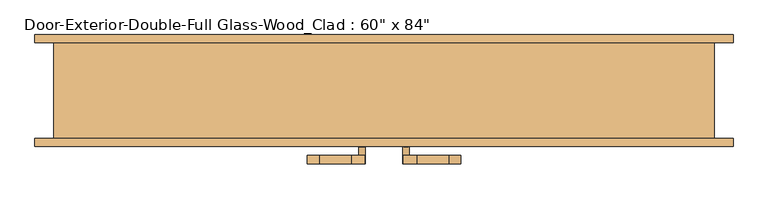
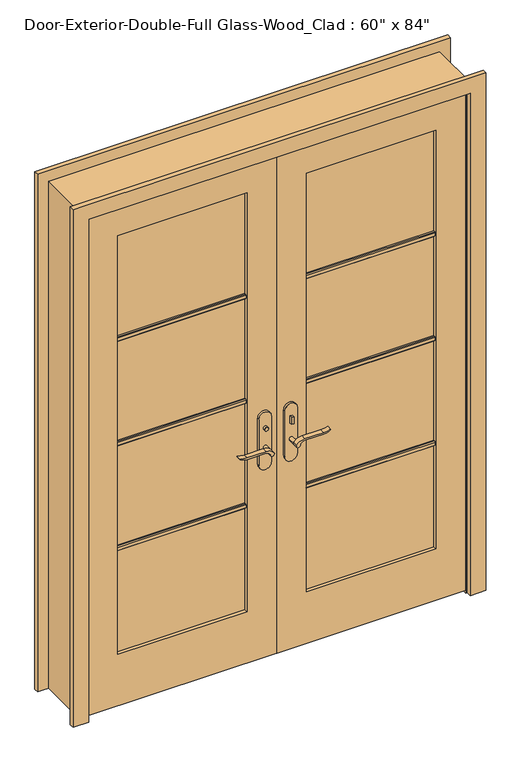
"""IFC4 building model written with IfcOpenShell, lengths in millimetres: door geometry."""

from ifc_helpers import new_model, si_unit, point, frame, frame_2d, origin, place, context, project, spatial, polyline, circle_curve, trimmed, segment, composite_curve, outline, extrude, faceted_brep, source, transform, mapped, element, save


def door_7bc300fe(model_context):
    return source(origin(), model_context, "Body", "SolidModel", [
        extrude(outline(polyline([(-19.05, 12.7), (6.35, 0.0), (-79.375, 0.0), (-53.975, 12.7), (-19.05, 12.7)])), frame((-762.0, 0.0, 0.0), z_axis=(1.0, 0.0, 0.0), x_axis=(0.0, 1.0, 0.0)), (0.0, 0.0, 1.0), 1524.0),
        extrude(outline(polyline([(-47.4019111, -56.2), (-47.4019111, -66.2), (-57.4019111, -66.2), (-57.4019111, -56.2), (-47.4019111, -56.2)])), frame((0.0, 0.0, 981.9), z_axis=(0.0, 0.0, 1.0), x_axis=(1.0, 0.0, 0.0)), (0.0, 0.0, 1.0), 30.0),
        extrude(outline(composite_curve([segment(trimmed(circle_curve(frame_2d((996.9, -52.4019111)), 8.0), [point((996.9, -60.4019111))], [point((996.9, -44.4019111))], False, "CARTESIAN"), True, "CONTINUOUS"), segment(trimmed(circle_curve(frame_2d((996.9, -52.4019111)), 8.0), [point((996.9, -44.4019111))], [point((996.9, -60.4019111))], False, "CARTESIAN"), True, "CONTINUOUS")], self_intersect=False)), frame((0.0, -131.125, 0.0), z_axis=(0.0, 1.0, 0.0), x_axis=(0.0, 0.0, 1.0)), (0.0, 0.0, 1.0), 10.0),
        extrude(outline(composite_curve([segment(trimmed(circle_curve(frame_2d((897.1555521, -76.0694241)), 37.2832219), [point((919.0523287, -45.8937749))], [point((934.4, -77.7693445))], False, "CARTESIAN"), True, "CONTINUOUS"), segment(polyline([(934.4, -77.7693445), (934.4, -154.045502)]), True, "CONTINUOUS"), segment(trimmed(circle_curve(frame_2d((1017.6850638, -153.9791202)), 83.2850902), [point((934.4, -154.045502))], [point((939.4, -182.4019111))], True, "CARTESIAN"), True, "CONTINUOUS"), segment(polyline([(939.4, -182.4019111), (936.6135558, -182.4019111)]), True, "CONTINUOUS"), segment(trimmed(circle_curve(frame_2d((986.6709207, -150.4622499)), 59.3791355), [point((936.6135558, -182.4019111))], [point((927.4, -154.045502))], False, "CARTESIAN"), True, "CONTINUOUS"), segment(polyline([(927.4, -154.045502), (927.4, -77.7881013)]), True, "CONTINUOUS"), segment(trimmed(circle_curve(frame_2d((909.2738613, -77.7881013)), 18.1261387), [point((927.4, -77.7881013))], [point((914.4, -60.4019111))], True, "CARTESIAN"), True, "CONTINUOUS"), segment(trimmed(circle_curve(frame_2d((914.4, -52.4019111)), 8.0), [point((914.4, -60.4019111))], [point((919.0523287, -45.8937749))], False, "CARTESIAN"), True, "CONTINUOUS")], self_intersect=False)), frame((0.0, -36.2, 0.0), z_axis=(0.0, 1.0, 0.0), x_axis=(0.0, 0.0, 1.0)), (0.0, 0.0, 1.0), 20.0),
        extrude(outline(composite_curve([segment(trimmed(circle_curve(frame_2d((914.4, -52.4019111)), 8.0), [point((914.3999903, -60.4019111))], [point((919.0523287, -45.8937749))], False, "CARTESIAN"), True, "CONTINUOUS"), segment(trimmed(circle_curve(frame_2d((897.1555521, -76.0694241)), 37.2832219), [point((919.0523287, -45.8937749))], [point((934.4, -77.7693445))], False, "CARTESIAN"), True, "CONTINUOUS"), segment(polyline([(934.4, -77.7693445), (934.4, -154.045502)]), True, "CONTINUOUS"), segment(trimmed(circle_curve(frame_2d((1017.6850638, -153.9791202)), 83.2850902), [point((934.4, -154.045502))], [point((939.4, -182.4019111))], True, "CARTESIAN"), True, "CONTINUOUS"), segment(polyline([(939.4, -182.4019111), (936.6135558, -182.4019111)]), True, "CONTINUOUS"), segment(trimmed(circle_curve(frame_2d((986.6709207, -150.4622499)), 59.3791355), [point((936.6135558, -182.4019111))], [point((927.4, -154.045502))], False, "CARTESIAN"), True, "CONTINUOUS"), segment(polyline([(927.4, -154.045502), (927.4, -77.788099)]), True, "CONTINUOUS"), segment(trimmed(circle_curve(frame_2d((909.2738682, -77.788099)), 18.1261318), [point((927.4, -77.788099))], [point((914.3999903, -60.4019111))], True, "CARTESIAN"), True, "CONTINUOUS")], self_intersect=False)), frame((0.0, -171.125, 0.0), z_axis=(0.0, 1.0, 0.0), x_axis=(0.0, 0.0, 1.0)), (0.0, 0.0, 1.0), 20.0),
        extrude(outline(composite_curve([segment(trimmed(circle_curve(frame_2d((914.4, -52.4019111)), 8.0), [point((914.4, -60.4019111))], [point((914.4, -44.4019111))], False, "CARTESIAN"), True, "CONTINUOUS"), segment(trimmed(circle_curve(frame_2d((914.4, -52.4019111)), 8.0), [point((914.4, -44.4019111))], [point((914.4, -60.4019111))], False, "CARTESIAN"), True, "CONTINUOUS")], self_intersect=False)), frame((0.0, -66.2, 0.0), z_axis=(0.0, 1.0, 0.0), x_axis=(0.0, 0.0, 1.0)), (0.0, 0.0, 1.0), 30.0),
        extrude(outline(composite_curve([segment(trimmed(circle_curve(frame_2d((914.4, -52.4019111)), 8.0), [point((914.4, -60.4019111))], [point((914.4, -44.4019111))], False, "CARTESIAN"), True, "CONTINUOUS"), segment(trimmed(circle_curve(frame_2d((914.4, -52.4019111)), 8.0), [point((914.4, -44.4019111))], [point((914.4, -60.4019111))], False, "CARTESIAN"), True, "CONTINUOUS")], self_intersect=False)), frame((0.0, -151.125, 0.0), z_axis=(0.0, 1.0, 0.0), x_axis=(0.0, 0.0, 1.0)), (0.0, 0.0, 1.0), 30.0),
        extrude(outline(composite_curve([segment(polyline([(844.4, -27.4019111), (1039.4, -27.4019111)]), True, "CONTINUOUS"), segment(trimmed(circle_curve(frame_2d((1039.4, -52.4019111)), 25.0), [point((1039.4, -27.4019111))], [point((1039.4, -77.4019111))], False, "CARTESIAN"), True, "CONTINUOUS"), segment(polyline([(1039.4, -77.4019111), (844.4, -77.4019111)]), True, "CONTINUOUS"), segment(trimmed(circle_curve(frame_2d((844.4, -52.4019111)), 25.0), [point((844.4, -77.4019111))], [point((844.4, -27.4019111))], False, "CARTESIAN"), True, "CONTINUOUS")], self_intersect=False)), frame((0.0, -76.2, 0.0), z_axis=(0.0, 1.0, 0.0), x_axis=(0.0, 0.0, 1.0)), (0.0, 0.0, 1.0), 10.0),
        extrude(outline(composite_curve([segment(polyline([(844.4, -27.4019111), (1039.4, -27.4019111)]), True, "CONTINUOUS"), segment(trimmed(circle_curve(frame_2d((1039.4, -52.4019111)), 25.0), [point((1039.4, -27.4019111))], [point((1039.4, -77.4019111))], False, "CARTESIAN"), True, "CONTINUOUS"), segment(polyline([(1039.4, -77.4019111), (844.4, -77.4019111)]), True, "CONTINUOUS"), segment(trimmed(circle_curve(frame_2d((844.4, -52.4019111)), 25.0), [point((844.4, -77.4019111))], [point((844.4, -27.4019111))], False, "CARTESIAN"), True, "CONTINUOUS")], self_intersect=False)), frame((0.0, -121.125, 0.0), z_axis=(0.0, 1.0, 0.0), x_axis=(0.0, 0.0, 1.0)), (0.0, 0.0, 1.0), 10.0),
        extrude(outline(polyline([(47.3875, -131.125), (47.3875, -121.125), (57.3875, -121.125), (57.3875, -131.125), (47.3875, -131.125)])), frame((0.0, 0.0, 981.9), z_axis=(0.0, 0.0, 1.0), x_axis=(1.0, 0.0, 0.0)), (0.0, 0.0, 1.0), 30.0),
        extrude(outline(composite_curve([segment(trimmed(circle_curve(frame_2d((996.9, 52.3875)), 8.0), [point((996.9, 60.3875))], [point((996.9, 44.3875))], False, "CARTESIAN"), True, "CONTINUOUS"), segment(trimmed(circle_curve(frame_2d((996.9, 52.3875)), 8.0), [point((996.9, 44.3875))], [point((996.9, 60.3875))], False, "CARTESIAN"), True, "CONTINUOUS")], self_intersect=False)), frame((0.0, -66.2, 0.0), z_axis=(0.0, 1.0, 0.0), x_axis=(0.0, 0.0, 1.0)), (0.0, 0.0, 1.0), 10.0),
        extrude(outline(composite_curve([segment(trimmed(circle_curve(frame_2d((914.4, 52.3875)), 8.0), [point((919.0523287, 45.8793637))], [point((914.4, 60.3875))], False, "CARTESIAN"), True, "CONTINUOUS"), segment(trimmed(circle_curve(frame_2d((909.2738613, 77.7736901)), 18.1261387), [point((914.4, 60.3875))], [point((927.4, 77.7736901))], True, "CARTESIAN"), True, "CONTINUOUS"), segment(polyline([(927.4, 77.7736901), (927.4, 154.0310909)]), True, "CONTINUOUS"), segment(trimmed(circle_curve(frame_2d((986.6709207, 150.4478388)), 59.3791355), [point((927.4, 154.0310909))], [point((936.6135558, 182.3875))], False, "CARTESIAN"), True, "CONTINUOUS"), segment(polyline([(936.6135558, 182.3875), (939.4, 182.3875)]), True, "CONTINUOUS"), segment(trimmed(circle_curve(frame_2d((1017.6850638, 153.9647091)), 83.2850902), [point((939.4, 182.3875))], [point((934.4, 154.0310909))], True, "CARTESIAN"), True, "CONTINUOUS"), segment(polyline([(934.4, 154.0310909), (934.4, 77.7549333)]), True, "CONTINUOUS"), segment(trimmed(circle_curve(frame_2d((897.1555521, 76.0550129)), 37.2832219), [point((934.4, 77.7549333))], [point((919.0523287, 45.8793637))], False, "CARTESIAN"), True, "CONTINUOUS")], self_intersect=False)), frame((0.0, -171.125, 0.0), z_axis=(0.0, 1.0, 0.0), x_axis=(0.0, 0.0, 1.0)), (0.0, 0.0, 1.0), 20.0),
        extrude(outline(composite_curve([segment(trimmed(circle_curve(frame_2d((909.2738682, 77.7736878)), 18.1261318), [point((914.3999903, 60.3875))], [point((927.4, 77.7736878))], True, "CARTESIAN"), True, "CONTINUOUS"), segment(polyline([(927.4, 77.7736878), (927.4, 154.0310909)]), True, "CONTINUOUS"), segment(trimmed(circle_curve(frame_2d((986.6709207, 150.4478388)), 59.3791355), [point((927.4, 154.0310909))], [point((936.6135558, 182.3875))], False, "CARTESIAN"), True, "CONTINUOUS"), segment(polyline([(936.6135558, 182.3875), (939.4, 182.3875)]), True, "CONTINUOUS"), segment(trimmed(circle_curve(frame_2d((1017.6850638, 153.9647091)), 83.2850902), [point((939.4, 182.3875))], [point((934.4, 154.0310909))], True, "CARTESIAN"), True, "CONTINUOUS"), segment(polyline([(934.4, 154.0310909), (934.4, 77.7549333)]), True, "CONTINUOUS"), segment(trimmed(circle_curve(frame_2d((897.1555521, 76.0550129)), 37.2832219), [point((934.4, 77.7549333))], [point((919.0523287, 45.8793637))], False, "CARTESIAN"), True, "CONTINUOUS"), segment(trimmed(circle_curve(frame_2d((914.4, 52.3875)), 8.0), [point((919.0523287, 45.8793637))], [point((914.3999903, 60.3875))], False, "CARTESIAN"), True, "CONTINUOUS")], self_intersect=False)), frame((0.0, -36.2, 0.0), z_axis=(0.0, 1.0, 0.0), x_axis=(0.0, 0.0, 1.0)), (0.0, 0.0, 1.0), 20.0),
        extrude(outline(composite_curve([segment(trimmed(circle_curve(frame_2d((914.4, 52.3875)), 8.0), [point((914.4, 60.3875))], [point((914.4, 44.3875))], False, "CARTESIAN"), True, "CONTINUOUS"), segment(trimmed(circle_curve(frame_2d((914.4, 52.3875)), 8.0), [point((914.4, 44.3875))], [point((914.4, 60.3875))], False, "CARTESIAN"), True, "CONTINUOUS")], self_intersect=False)), frame((0.0, -151.125, 0.0), z_axis=(0.0, 1.0, 0.0), x_axis=(0.0, 0.0, 1.0)), (0.0, 0.0, 1.0), 30.0),
        extrude(outline(composite_curve([segment(trimmed(circle_curve(frame_2d((914.4, 52.3875)), 8.0), [point((914.4, 60.3875))], [point((914.4, 44.3875))], False, "CARTESIAN"), True, "CONTINUOUS"), segment(trimmed(circle_curve(frame_2d((914.4, 52.3875)), 8.0), [point((914.4, 44.3875))], [point((914.4, 60.3875))], False, "CARTESIAN"), True, "CONTINUOUS")], self_intersect=False)), frame((0.0, -66.2, 0.0), z_axis=(0.0, 1.0, 0.0), x_axis=(0.0, 0.0, 1.0)), (0.0, 0.0, 1.0), 30.0),
        extrude(outline(composite_curve([segment(trimmed(circle_curve(frame_2d((844.4, 52.3875)), 25.0), [point((844.4, 27.3875))], [point((844.4, 77.3875))], False, "CARTESIAN"), True, "CONTINUOUS"), segment(polyline([(844.4, 77.3875), (1039.4, 77.3875)]), True, "CONTINUOUS"), segment(trimmed(circle_curve(frame_2d((1039.4, 52.3875)), 25.0), [point((1039.4, 77.3875))], [point((1039.4, 27.3875))], False, "CARTESIAN"), True, "CONTINUOUS"), segment(polyline([(1039.4, 27.3875), (844.4, 27.3875)]), True, "CONTINUOUS")], self_intersect=False)), frame((0.0, -121.125, 0.0), z_axis=(0.0, 1.0, 0.0), x_axis=(0.0, 0.0, 1.0)), (0.0, 0.0, 1.0), 10.0),
        extrude(outline(composite_curve([segment(trimmed(circle_curve(frame_2d((844.4, 52.3875)), 25.0), [point((844.4, 27.3875))], [point((844.4, 77.3875))], False, "CARTESIAN"), True, "CONTINUOUS"), segment(polyline([(844.4, 77.3875), (1039.4, 77.3875)]), True, "CONTINUOUS"), segment(trimmed(circle_curve(frame_2d((1039.4, 52.3875)), 25.0), [point((1039.4, 77.3875))], [point((1039.4, 27.3875))], False, "CARTESIAN"), True, "CONTINUOUS"), segment(polyline([(1039.4, 27.3875), (844.4, 27.3875)]), True, "CONTINUOUS")], self_intersect=False)), frame((0.0, -76.2, 0.0), z_axis=(0.0, 1.0, 0.0), x_axis=(0.0, 0.0, 1.0)), (0.0, 0.0, 1.0), 10.0),
        extrude(outline(polyline([(-90.17, 1578.371875), (-83.82, 1578.371875), (-80.645, 1575.196875), (-80.645, 1562.496875), (-83.82, 1559.321875), (-90.17, 1559.321875), (-90.17, 1578.371875)])), frame((120.65, 0.0, 0.0), z_axis=(1.0, 0.0, 0.0), x_axis=(0.0, 1.0, 0.0)), (0.0, 0.0, 1.0), 520.7),
        extrude(outline(polyline([(-90.17, 1132.68125), (-83.82, 1132.68125), (-80.645, 1129.50625), (-80.645, 1116.80625), (-83.82, 1113.63125), (-90.17, 1113.63125), (-90.17, 1132.68125)])), frame((120.65, 0.0, 0.0), z_axis=(1.0, 0.0, 0.0), x_axis=(0.0, 1.0, 0.0)), (0.0, 0.0, 1.0), 520.7),
        extrude(outline(polyline([(-90.17, 686.990625), (-83.82, 686.990625), (-80.645, 683.815625), (-80.645, 671.115625), (-83.82, 667.940625), (-90.17, 667.940625), (-90.17, 686.990625)])), frame((120.65, 0.0, 0.0), z_axis=(1.0, 0.0, 0.0), x_axis=(0.0, 1.0, 0.0)), (0.0, 0.0, 1.0), 520.7),
        extrude(outline(polyline([(-97.155, 1578.371875), (-97.155, 1559.321875), (-103.505, 1559.321875), (-106.68, 1562.496875), (-106.68, 1575.196875), (-103.505, 1578.371875), (-97.155, 1578.371875)])), frame((-641.35, 0.0, 0.0), z_axis=(1.0, 0.0, 0.0), x_axis=(0.0, 1.0, 0.0)), (0.0, 0.0, 1.0), 520.7),
        extrude(outline(polyline([(-97.155, 1132.68125), (-97.155, 1113.63125), (-103.505, 1113.63125), (-106.68, 1116.80625), (-106.68, 1129.50625), (-103.505, 1132.68125), (-97.155, 1132.68125)])), frame((-641.35, 0.0, 0.0), z_axis=(1.0, 0.0, 0.0), x_axis=(0.0, 1.0, 0.0)), (0.0, 0.0, 1.0), 520.7),
        extrude(outline(polyline([(-97.155, 686.990625), (-97.155, 667.940625), (-103.505, 667.940625), (-106.68, 671.115625), (-106.68, 683.815625), (-103.505, 686.990625), (-97.155, 686.990625)])), frame((-641.35, 0.0, 0.0), z_axis=(1.0, 0.0, 0.0), x_axis=(0.0, 1.0, 0.0)), (0.0, 0.0, 1.0), 520.7),
        extrude(outline(polyline([(-97.155, 1578.371875), (-97.155, 1559.321875), (-103.505, 1559.321875), (-106.68, 1562.496875), (-106.68, 1575.196875), (-103.505, 1578.371875), (-97.155, 1578.371875)])), frame((120.65, 0.0, 0.0), z_axis=(1.0, 0.0, 0.0), x_axis=(0.0, 1.0, 0.0)), (0.0, 0.0, 1.0), 520.7),
        extrude(outline(polyline([(-97.155, 1132.68125), (-97.155, 1113.63125), (-103.505, 1113.63125), (-106.68, 1116.80625), (-106.68, 1129.50625), (-103.505, 1132.68125), (-97.155, 1132.68125)])), frame((120.65, 0.0, 0.0), z_axis=(1.0, 0.0, 0.0), x_axis=(0.0, 1.0, 0.0)), (0.0, 0.0, 1.0), 520.7),
        extrude(outline(polyline([(-97.155, 686.990625), (-97.155, 667.940625), (-103.505, 667.940625), (-106.68, 671.115625), (-106.68, 683.815625), (-103.505, 686.990625), (-97.155, 686.990625)])), frame((120.65, 0.0, 0.0), z_axis=(1.0, 0.0, 0.0), x_axis=(0.0, 1.0, 0.0)), (0.0, 0.0, 1.0), 520.7),
        extrude(outline(polyline([(-90.17, 1578.371875), (-83.82, 1578.371875), (-80.645, 1575.196875), (-80.645, 1562.496875), (-83.82, 1559.321875), (-90.17, 1559.321875), (-90.17, 1578.371875)])), frame((-641.35, 0.0, 0.0), z_axis=(1.0, 0.0, 0.0), x_axis=(0.0, 1.0, 0.0)), (0.0, 0.0, 1.0), 520.7),
        extrude(outline(polyline([(-90.17, 1132.68125), (-83.82, 1132.68125), (-80.645, 1129.50625), (-80.645, 1116.80625), (-83.82, 1113.63125), (-90.17, 1113.63125), (-90.17, 1132.68125)])), frame((-641.35, 0.0, 0.0), z_axis=(1.0, 0.0, 0.0), x_axis=(0.0, 1.0, 0.0)), (0.0, 0.0, 1.0), 520.7),
        extrude(outline(polyline([(-90.17, 686.990625), (-83.82, 686.990625), (-80.645, 683.815625), (-80.645, 671.115625), (-83.82, 667.940625), (-90.17, 667.940625), (-90.17, 686.990625)])), frame((-641.35, 0.0, 0.0), z_axis=(1.0, 0.0, 0.0), x_axis=(0.0, 1.0, 0.0)), (0.0, 0.0, 1.0), 520.7),
        extrude(outline(polyline([(0.0, 831.85), (2203.45, 831.85), (2203.45, -831.85), (0.0, -831.85), (0.0, -768.35), (2139.95, -768.35), (2139.95, 768.35), (0.0, 768.35), (0.0, 831.85)])), frame((0.0, 117.475, 0.0), z_axis=(0.0, 1.0, 0.0), x_axis=(0.0, 0.0, 1.0)), (0.0, 0.0, 1.0), 19.05),
        extrude(outline(polyline([(0.0, 831.85), (2203.45, 831.85), (2203.45, -831.85), (0.0, -831.85), (0.0, -768.35), (2139.95, -768.35), (2139.95, 768.35), (0.0, 768.35), (0.0, 831.85)])), frame((0.0, -130.175, 0.0), z_axis=(0.0, 1.0, 0.0), x_axis=(0.0, 0.0, 1.0)), (0.0, 0.0, 1.0), 19.05),
        faceted_brep([(787.4, -111.125, 0.0), (762.0, -111.125, 0.0), (762.0, -76.2, 0.0), (749.3, -76.2, 0.0), (749.3, -41.275, 0.0), (762.0, -41.275, 0.0), (762.0, 117.475, 0.0), (787.4, 117.475, 0.0), (787.4, 117.475, 2159.0), (787.4, -111.125, 2159.0), (762.0, 117.475, 2133.6), (-762.0, 117.475, 2133.6), (-762.0, 117.475, 0.0), (-787.4, 117.475, 0.0), (-787.4, 117.475, 2159.0), (762.0, -41.275, 2133.6), (749.3, -41.275, 2120.9), (-749.3, -41.275, 2120.9), (-749.3, -41.275, 0.0), (-762.0, -41.275, 0.0), (-762.0, -41.275, 2133.6), (749.3, -76.2, 2120.9), (762.0, -76.2, 2133.6), (1.5875, -76.2, 2133.6), (-1.6019111, -76.2, 2133.6), (-762.0, -76.2, 2133.6), (-762.0, -76.2, 0.0), (-749.3, -76.2, 0.0), (-749.3, -76.2, 2120.9), (-1.6019111, -76.2, 2120.9), (1.5875, -76.2, 2120.9), (762.0, -111.125, 2133.6), (-787.4, -111.125, 2159.0), (-787.4, -111.125, 0.0), (-762.0, -111.125, 0.0), (-762.0, -111.125, 2133.6), (-1.6019111, -111.125, 2133.6), (1.5875, -111.125, 2133.6)], [[[0, 1, 2, 3, 4, 5, 6, 7]], [[7, 8, 9, 0]], [[6, 10, 11, 12, 13, 14, 8, 7]], [[5, 15, 10, 6]], [[4, 16, 17, 18, 19, 20, 15, 5]], [[3, 21, 16, 4]], [[2, 22, 23, 24, 25, 26, 27, 28, 29, 30, 21, 3]], [[1, 31, 22, 2]], [[0, 9, 32, 33, 34, 35, 36, 37, 31, 1]], [[8, 14, 32, 9]], [[10, 15, 20, 11]], [[16, 21, 30, 29, 28, 17]], [[31, 37, 36, 35, 25, 24, 23, 22]], [[12, 19, 18, 27, 26, 34, 33, 13]], [[13, 33, 32, 14]], [[11, 20, 19, 12]], [[17, 28, 27, 18]], [[25, 35, 34, 26]]]),
        extrude(outline(polyline([(2133.6, 762.0), (2133.6, 1.5875), (12.7, 1.5875), (12.7, 762.0), (2133.6, 762.0)]), holes=[polyline([(2014.5375, 120.65), (2014.5375, 641.35), (231.775, 641.35), (231.775, 120.65), (2014.5375, 120.65)])]), frame((0.0, -111.125, 0.0), z_axis=(0.0, 1.0, 0.0), x_axis=(0.0, 0.0, 1.0)), (0.0, 0.0, 1.0), 34.925),
        extrude(outline(polyline([(12.7, -762.0), (12.7, -1.6019111), (2133.6, -1.6019111), (2133.6, -762.0), (12.7, -762.0)]), holes=[polyline([(231.775, -641.35), (2014.5375, -641.35), (2014.5375, -120.65), (231.775, -120.65), (231.775, -641.35)])]), frame((0.0, -111.125, 0.0), z_axis=(0.0, 1.0, 0.0), x_axis=(0.0, 0.0, 1.0)), (0.0, 0.0, 1.0), 34.925),
        extrude(outline(polyline([(641.35, -90.17), (641.35, -97.155), (120.65, -97.155), (120.65, -90.17), (641.35, -90.17)])), frame((0.0, 0.0, 231.775), z_axis=(0.0, 0.0, 1.0), x_axis=(1.0, 0.0, 0.0)), (0.0, 0.0, 1.0), 1782.7625),
        extrude(outline(polyline([(-120.65, -90.17), (-120.65, -97.155), (-641.35, -97.155), (-641.35, -90.17), (-120.65, -90.17)])), frame((0.0, 0.0, 231.775), z_axis=(0.0, 0.0, 1.0), x_axis=(1.0, 0.0, 0.0)), (0.0, 0.0, 1.0), 1782.7625),
    ])


if __name__ == "__main__":
    model = new_model("IFC4")
    model_context = context("Model", 3, world=origin())
    ifc_project = project(units=[si_unit("LENGTHUNIT", "METRE", prefix="MILLI")], contexts=[model_context])
    site = spatial("IfcSite", under=ifc_project)
    building = spatial("IfcBuilding", under=site)
    placement = place(None, origin())
    door_shape = door_7bc300fe(model_context)
    element("IfcDoor", 1, ObjectType="Door-Exterior-Double-Full Glass-Wood_Clad : 60\" x 84\"", at=placement, inside=building, context=model_context, shape_type="MappedRepresentation", body=[
        mapped(door_shape, transform((0.0, 0.0, 0.0), x_axis=(1.0, 0.0, 0.0), y_axis=(0.0, 1.0, 0.0), z_axis=(0.0, 0.0, 1.0))),
    ])
    save(model, "model.ifc")

# Revit data of these elements
# Type "Door-Exterior-Double-Full Glass-Wood_Clad : 60\" x 84\""
#   Type Mark = "9"
#   Assembly Code = "B2030100"
#   Analytic Construction = "French door, wood frame with double glass"
#   Top Rail = 0' - 4 11/16"
#   Threshold Offset [instance default] = 0' - 0 1/2"
#   Thickness = 0' - 1 3/8"
#   Thermal Resistance (R) = 1.9158 (h·ft²·°F)/BTU
#   Swing Angle [instance default] = 90.00°
#   Stiles = 0' - 4 3/4"
#   Rough Width = 5' - 2"
#   Rough Height = 7' - 1"
#   Panel Width = 2' - 6"
#   Door Offset [instance default] = 0' - 0"
#   Height = 7' - 0"
#   Width = 5' - 0"
#   Heat Transfer Coefficient (U) = 0.5220 BTU/(h·ft²·°F)
#   Bottom Rail = 0' - 9 1/8"
#   Exterior Trim [instance default] = yes
#   Threshold [instance default] = yes
#   Show Grill [instance default] = yes
#   Function = 1
#   Trim Material = Cherry
#   Threshold Material = Cherry
#   Panel Material = Cherry
#   Glazing = Glass
#   Frame Material = Cherry
#   Door Handle Material = Aluminum
#   Visual Light Transmittance = 0
#   Solar Heat Gain Coefficient = 0
#   Wall Closure = (empty or 0)
#   Construction Type = (empty or 0)
# Element 1 (IfcDoor, "Door-Exterior-Double-Full Glass-Wood_Clad : 60\" x 84\"")
#   Materials on its faces: "Cherry", "Aluminum", "Glass"
# Materials
#   "Cherry": class "Wood", colour RGB 226 177 128, transparency 0, Description = "Prunus Serotina", Cost = 0
#   "Glass": class "Glass", colour RGB 0 128 192, transparency 0.75, Description = "Soda Lime Glass", Cost = 0
#   "Aluminum": class "Metal", colour RGB 247 247 247, transparency 0, Description = "Aluminum 6061", Cost = 0
